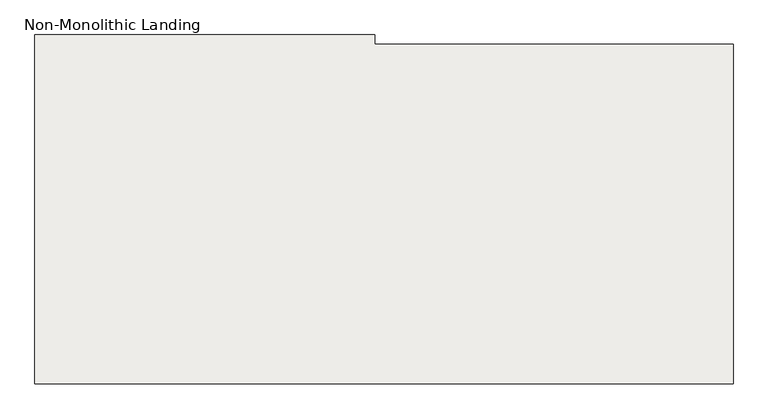
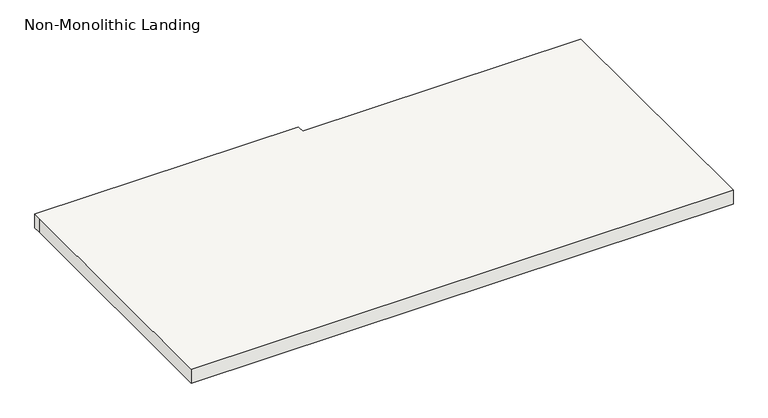
"""IFC4 building model written with IfcOpenShell, lengths in millimetres: slab geometry, Non-Monolithic Landing."""

from ifc_helpers import new_model, si_unit, origin, place, context, project, spatial, faceted_brep, source, transform, mapped, element, save


def non_monolithic_landing_7b61c384(model_context):
    return source(origin(), model_context, "Body", "Brep", [
        faceted_brep([(-3400.7137331, -6527.0593836, 4705.35), (-3400.7137331, -6552.4593836, 4679.95), (-4315.1137331, -6552.4593836, 4679.95), (-4315.1137331, -6527.0593836, 4705.35), (-4365.9137331, -6527.0593836, 4724.4), (-4365.9137331, -6501.6593836, 4724.4), (-5280.3137331, -6501.6593836, 4724.4), (-5280.3137331, -6527.0593836, 4724.4), (-5280.3137331, -7441.4593836, 4724.4), (-3400.7137331, -7441.4593836, 4724.4), (-3400.7137331, -6527.0593836, 4724.4), (-4315.1137331, -6552.4593836, 4673.6), (-3400.7137331, -6552.4593836, 4673.6), (-3400.7137331, -7441.4593836, 4673.6), (-5280.3137331, -7441.4593836, 4673.6), (-5280.3137331, -6527.0593836, 4673.6), (-5280.3137331, -6501.6593836, 4673.6), (-4365.9137331, -6501.6593836, 4673.6), (-4365.9137331, -6527.0593836, 4673.6), (-4315.1137331, -6527.0593836, 4673.6)], [[[0, 1, 2, 3]], [[4, 5, 6, 7, 8, 9, 10]], [[11, 12, 13, 14, 15, 16, 17, 18, 19]], [[12, 11, 2, 1]], [[11, 19, 3, 2]], [[4, 10, 0, 3, 19, 18]], [[5, 4, 18, 17]], [[6, 5, 17, 16]], [[7, 6, 16, 15]], [[8, 7, 15, 14]], [[9, 8, 14, 13]], [[10, 9, 13, 12, 1, 0]]]),
    ])


if __name__ == "__main__":
    model = new_model("IFC4")
    model_context = context("Model", 3, world=origin())
    ifc_project = project(units=[si_unit("LENGTHUNIT", "METRE", prefix="MILLI")], contexts=[model_context])
    site = spatial("IfcSite", under=ifc_project)
    building = spatial("IfcBuilding", under=site)
    placement = place(None, origin())
    non_monolithic_landing_shape = non_monolithic_landing_7b61c384(model_context)
    element("IfcSlab", 1, ObjectType="Non-Monolithic Landing", at=placement, inside=building, context=model_context, shape_type="MappedRepresentation", body=[
        mapped(non_monolithic_landing_shape, transform((0.0, 0.0, 0.0), x_axis=(1.0, 0.0, 0.0), y_axis=(0.0, 1.0, 0.0), z_axis=(0.0, 0.0, 1.0))),
    ])
    save(model, "model.ifc")
